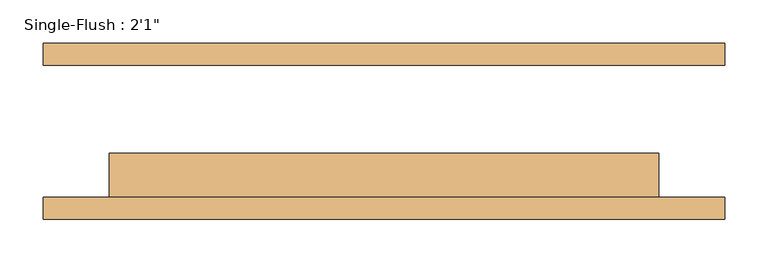
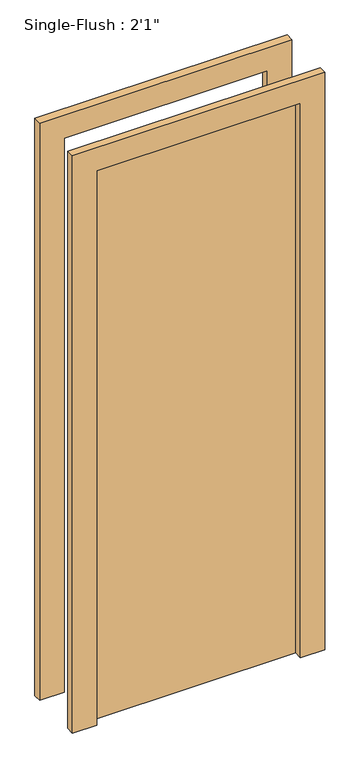
"""IFC4 building model written with IfcOpenShell, lengths in millimetres: door geometry."""

from ifc_helpers import new_model, si_unit, frame, origin, origin_with_axes, place, context, project, spatial, polyline, outline, extrude, source, transform, mapped, element, save


def door_fe267433(model_context):
    return source(origin(), model_context, "Body", "SweptSolid", [
        extrude(outline(polyline([(1905.0, -393.7), (0.0, -393.7), (0.0, -317.5), (1828.8, -317.5), (1828.8, 317.5), (0.0, 317.5), (0.0, 393.7), (1905.0, 393.7), (1905.0, -393.7)])), frame((0.0, -101.6, 0.0), z_axis=(0.0, 1.0, 0.0), x_axis=(0.0, 0.0, 1.0)), (0.0, 0.0, 1.0), 25.4),
        extrude(outline(polyline([(1905.0, 393.7), (1905.0, -393.7), (0.0, -393.7), (0.0, -317.5), (1828.8, -317.5), (1828.8, 317.5), (0.0, 317.5), (0.0, 393.7), (1905.0, 393.7)])), frame((0.0, 76.2, 0.0), z_axis=(0.0, 1.0, 0.0), x_axis=(0.0, 0.0, 1.0)), (0.0, 0.0, 1.0), 25.4),
        extrude(outline(polyline([(317.5, -25.4), (317.5, -76.2), (-317.5, -76.2), (-317.5, -25.4), (317.5, -25.4)])), origin_with_axes(), (0.0, 0.0, 1.0), 1828.8),
    ])


if __name__ == "__main__":
    model = new_model("IFC4")
    model_context = context("Model", 3, world=origin())
    ifc_project = project(units=[si_unit("LENGTHUNIT", "METRE", prefix="MILLI")], contexts=[model_context])
    site = spatial("IfcSite", under=ifc_project)
    building = spatial("IfcBuilding", under=site)
    placement = place(None, origin())
    door_shape = door_fe267433(model_context)
    element("IfcDoor", 1, ObjectType="Single-Flush : 2'1\"", at=placement, inside=building, context=model_context, shape_type="MappedRepresentation", body=[
        mapped(door_shape, transform((0.0, 0.0, 0.0), x_axis=(1.0, 0.0, 0.0), y_axis=(0.0, 1.0, 0.0), z_axis=(0.0, 0.0, 1.0))),
    ])
    save(model, "model.ifc")

# Revit data of these elements
# Type "Single-Flush : 2'1\""
#   Type Mark = "9"
#   Construction Type Id = "MDOOR"
#   Assembly Code = "C1020"
#   Analytic Construction = "Metal"
#   Thickness = 0' - 2"
#   Heat Transfer Coefficient (U) = 0.651978 BTU/(h·ft²·°F)
#   Height = 6' - 0"
#   Trim Projection Ext = 0' - 1"
#   Trim Projection Int = 0' - 1"
#   Trim Width = 0' - 3"
#   Width = 2' - 1"
#   Define Thermal Properties by = 1
#   Door Material = Door - Panel
#   Frame Material = Door - Frame
#   Visual Light Transmittance = 0
#   Solar Heat Gain Coefficient = 0
#   Function = (empty or 0)
#   Wall Closure = (empty or 0)
# Element 1 (IfcDoor, "Single-Flush : 2'1\"")
#   Materials on its faces: "Door - Frame", "Door - Panel"
# Materials
#   "Door - Panel": class "Wood", colour RGB 210 159 95, transparency 0, Cost = 0
#   "Door - Frame": colour RGB 118 70 51, transparency 0, Cost = 0
